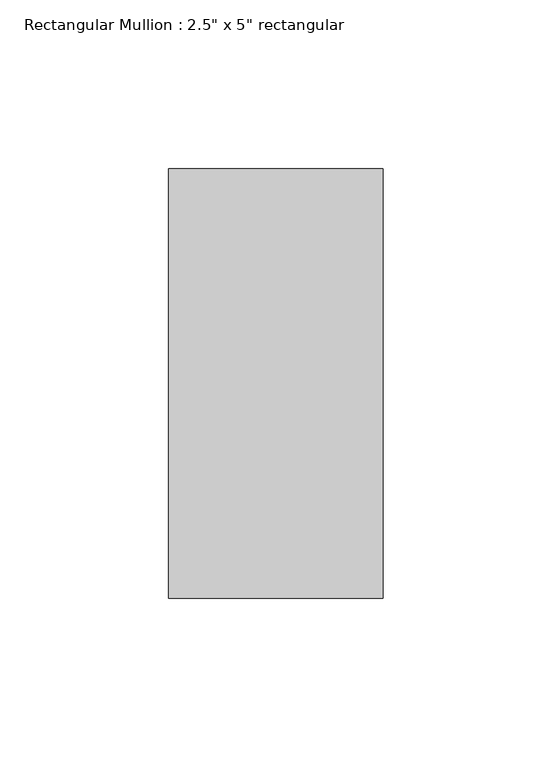
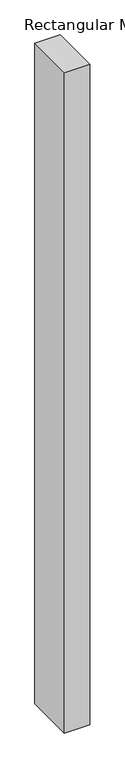
"""IFC4 building model written with IfcOpenShell, lengths in millimetres: member geometry."""

from ifc_helpers import new_model, si_unit, frame, origin, place, context, project, spatial, polyline, outline, extrude, source, transform, mapped, element, save


def member_82128145(model_context):
    return source(origin(), model_context, "Body", "SweptSolid", [
        extrude(outline(polyline([(0.0, 63.5), (0.0, -63.5), (-63.5, -63.5), (-63.5, 63.5), (0.0, 63.5)])), frame((0.0, 0.0, -1736.1531464), z_axis=(0.0, 0.0, 1.0), x_axis=(1.0, 0.0, 0.0)), (0.0, 0.0, 1.0), 1736.1531464),
    ])


if __name__ == "__main__":
    model = new_model("IFC4")
    model_context = context("Model", 3, world=origin())
    ifc_project = project(units=[si_unit("LENGTHUNIT", "METRE", prefix="MILLI")], contexts=[model_context])
    site = spatial("IfcSite", under=ifc_project)
    building = spatial("IfcBuilding", under=site)
    placement = place(None, origin())
    member_shape = member_82128145(model_context)
    element("IfcMember", 1, ObjectType="Rectangular Mullion : 2.5\" x 5\" rectangular", at=placement, inside=building, context=model_context, shape_type="MappedRepresentation", body=[
        mapped(member_shape, transform((0.0, 0.0, 0.0), x_axis=(1.0, 0.0, 0.0), y_axis=(0.0, 1.0, 0.0), z_axis=(0.0, 0.0, 1.0))),
    ])
    save(model, "model.ifc")

# Revit data of these elements
# Type "Rectangular Mullion : 2.5\" x 5\" rectangular"
#   built-in parameter 1007304 = 0.416667 (stored number, unit not read)
#   built-in parameter 1007301 = 0.104167 (stored number, unit not read)
#   built-in parameter 1007300 = 0.104167 (stored number, unit not read)
# Element 1 (IfcMember, "Rectangular Mullion : 2.5\" x 5\" rectangular")
#   Materials on its faces: "Aluminum"
# Materials
#   "Aluminum": class "Metal", colour RGB 247 247 247, transparency 0, Description = "Aluminum 6061", Cost = 0
